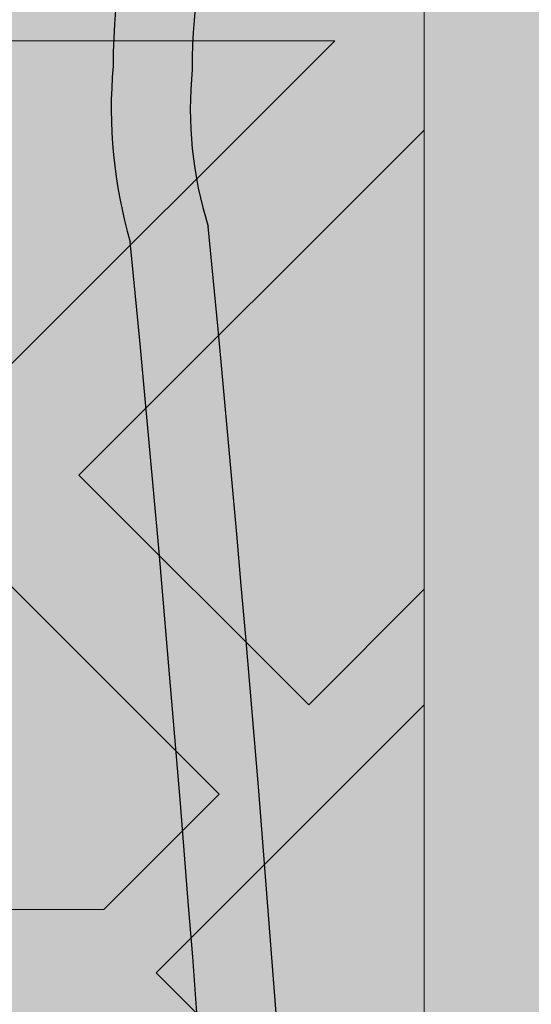
# Model space of a CAD drawing. Units: inches. Extents: x 844 to 2234, y 346 to 1084.
# Tile 20 of 93: x 1126.504 to 1127.536, y 701.258 to 703.246. Entities that reach past the tile are written whole.
import ezdxf

# ---------------------------------------------------------------- set-up
doc = ezdxf.new("R2010")
doc.units = ezdxf.units.IN
doc.header["$MEASUREMENT"] = 0
for name, color, linetype, lineweight in [('A-ANNO-DIMS', 2, 'Continuous', 18), ('furniture', 8, 'Continuous', 18), ('RA-AP-01$0$INT', 35, 'Continuous', 5)]:
    doc.layers.add(name, color=color, linetype=linetype, lineweight=lineweight)
doc.layers.add('RA-AP-01$0$FURN', color=3, linetype='Continuous')
doc.layers.add('RA-AP-01$0$WOOD', color=64, linetype='Continuous')
doc.styles.get("Standard").update_dxf_attribs({"font": 'arial.ttf'})
doc.dimstyles.get("Standard").update_dxf_attribs({"dimtxt": 6, "dimasz": 3, "dimexe": 0.18, "dimexo": 0.0625, "dimgap": 0.09, "dimtad": 0, "dimtih": 1, "dimtoh": 1, "dimdec": 1, "dimzin": 0, "dimdsep": 46, "dimlunit": 3, "dimtxsty": 'Standard', "dimblk": 'ARCHTICK', "dimcen": 0.09, "dimadec": 0, "dimazin": 0, "dimtfac": 1, "dimtdec": 1, "dimtofl": 0, "dimtmove": 0, "dimatfit": 3, "dimfxl": 1, "dimtolj": 1, "dimtzin": 0, "dimarcsym": 0})

# ---------------------------------------------------------------- blocks, each defined once
blk = doc.blocks.new('A$C18D01794')
at = {"layer": 'RA-AP-01$0$INT'}
blk.add_hatch(color=256, dxfattribs=at).paths.add_polyline_path([(4.505206456958071, -7.906712009588039), (5.305206456958072, -7.906712009588039), (5.305206456958072, -7.106712009588038), (5.255206456951893, -7.106712009588036), (5.25520645694868, -7.856712009570104), (4.555206456959269, -7.856712009588616), (4.555206456956052, -7.106712009588038), (4.505206456958073, -7.106712009588038)])
h = blk.add_hatch(color=256, dxfattribs=at)
h.paths.add_polyline_path([(4.585917135068448, -7.856712009587804), (4.614201406330596, -7.856712009587056), (4.668846067270487, -7.802067348644738), (4.723490728212344, -7.856712009584164), (4.771774999457151, -7.856712009582887), (4.826419660396886, -7.80206734864072), (4.862780050090322, -7.838427738332541), (4.844495778842715, -7.856712009580965), (4.862780050090411, -7.856712009580482), (4.905206456960182, -7.814285602707865), (4.947632863832445, -7.856712009578238), (4.965917135079675, -7.856712009577755), (4.947632863831759, -7.838427738330656), (4.983993253523576, -7.802067348637219), (5.038637914464627, -7.856712009575829), (5.08692218571208, -7.856712009574554), (5.141566846649976, -7.802067348634224), (5.196211507589851, -7.856712009571666), (5.224495778822615, -7.856712009570916), (4.905206456953975, -7.537422687702283)])
h.paths.add_polyline_path([(4.895206456956031, -7.575706958950402), (4.895206456958921, -7.684996280828174), (4.840561796018589, -7.630351619890275)], flags=16)
h.paths.add_polyline_path([(4.915206456955638, -7.575706958949956), (4.969851117895509, -7.630351619887399), (4.915206456957609, -7.684996280827732)], flags=16)
h.paths.add_polyline_path([(4.826419660395175, -7.644493755514321), (4.881064321335613, -7.699138416452331), (4.771774999456703, -7.69913841645522)], flags=16)
h.paths.add_polyline_path([(4.983993253519558, -7.644493755510815), (5.038637914460456, -7.699138416449285), (4.929348592581548, -7.69913841645126)], flags=16)
h.paths.add_polyline_path([(4.881064321336025, -7.719138416452334), (4.826419660397532, -7.773783077393256), (4.771774999457062, -7.719138416455217)], flags=16)
h.paths.add_polyline_path([(4.929348592582019, -7.71913841645126), (5.038637914460982, -7.719138416449284), (4.983993253522945, -7.773783077389749)], flags=16)
h.paths.add_polyline_path([(4.895206456960191, -7.733280552075633), (4.895206456962115, -7.806001331460164), (4.876922185715016, -7.824285602708492), (4.840561796021581, -7.787925213016675)], flags=16)
h.paths.add_polyline_path([(4.915206456958487, -7.733280552075187), (4.969851117899527, -7.787925213013798), (4.933490728206909, -7.824285602708034), (4.9152064569598, -7.806001331461736)], flags=16)
h.paths.add_polyline_path([(4.757632863832376, -7.733280552079264), (4.812277524772842, -7.787925213017304), (4.757632863834348, -7.842569873958233)], flags=16)
h.paths.add_polyline_path([(4.737632863832376, -7.73328055207979), (4.737632863834348, -7.842569873958701), (4.682988202893906, -7.787925213020692)], flags=16)
h.paths.add_polyline_path([(5.05278005008503, -7.733280552072701), (5.052780050087917, -7.842569873951664), (4.998135389146995, -7.787925213013169)], flags=16)
h.paths.add_polyline_path([(5.072780050085024, -7.733280552072333), (5.127424711025931, -7.787925213010806), (5.072780050087916, -7.842569873951244)], flags=16)
h.paths.add_polyline_path([(4.935917135072783, -7.506712009583784), (5.255206456948811, -7.826001331459767), (5.255206456948932, -7.797717060211899), (5.200561796010279, -7.743072399273238), (5.255206456949403, -7.688427738334128), (5.25520645694961, -7.640143467086677), (5.200561796009787, -7.585498806146837), (5.236922185702417, -7.549138416454212), (5.255206456949919, -7.56742268770172), (5.255206456949998, -7.549138416454178), (5.212780050078687, -7.506712009583814), (5.25520645695036, -7.464285602712145), (5.255206456950438, -7.446001331464763), (5.236922185702424, -7.464285602712779), (5.200561796009796, -7.427925213020149), (5.255206456950753, -7.373280552079203), (5.25520645695096, -7.324996280834394), (5.200561796010322, -7.270351619893748), (5.255206456951428, -7.215706958952649), (5.255206456951547, -7.187422687705071)])
h.paths.add_polyline_path([(5.042988202883395, -7.42792521302065), (5.097632863823085, -7.373280552080975), (5.097632863822622, -7.482569873959883)], flags=16)
h.paths.add_polyline_path([(5.028846067259663, -7.442067348644384), (5.083490728198774, -7.496712009583504), (4.974201406321001, -7.496712009583035)], flags=16)
h.paths.add_polyline_path([(5.117632863823087, -7.37328055208089), (5.172277524762331, -7.42792521302015), (5.11763286382262, -7.482569873959851)], flags=16)
h.paths.add_polyline_path([(5.08349072819877, -7.516712009582191), (5.028846067259652, -7.571356670521302), (4.974201406320998, -7.516712009582638)], flags=16)
h.paths.add_polyline_path([(5.131774999446817, -7.35913841645716), (5.186419660386065, -7.413783077396415), (5.241064321325782, -7.359138416456712)], flags=17)
h.paths.add_polyline_path([(5.131774999446228, -7.496712009583703), (5.186419660386065, -7.442067348643883), (5.222780050079488, -7.478427738337313), (5.204495778832781, -7.496712009584014)], flags=16)
h.paths.add_polyline_path([(5.097632863822613, -7.530854145205813), (5.097632863823061, -7.640143467084723), (5.042988202883383, -7.585498806145032)], flags=16)
h.paths.add_polyline_path([(5.131774999446899, -7.339138416457162), (5.241064321325809, -7.339138416456712), (5.186419660386591, -7.284493755517479)], flags=17)
h.paths.add_polyline_path([(5.131774999446226, -7.516712009581999), (5.204495778830767, -7.516712009581702), (5.22278005007868, -7.534996280829206), (5.186419660386049, -7.571356670521828)], flags=16)
h.paths.add_polyline_path([(5.11763286382262, -7.530854145205852), (5.17227752476232, -7.585498806145562), (5.117632863823064, -7.64014346708481)], flags=16)
h.paths.add_polyline_path([(5.186419660386069, -7.599640941770585), (5.241064321325754, -7.654285602710281), (5.131774999446791, -7.654285602709814)], flags=16)
h.paths.add_polyline_path([(5.131774999446872, -7.674285602709813), (5.24106432132578, -7.674285602710282), (5.186419660386554, -7.728930263649504)], flags=16)
h.paths.add_polyline_path([(5.255206456951811, -7.126001331467467), (5.255206456951895, -7.106712009588038), (4.555206456956052, -7.106712009588038), (4.555206456956136, -7.12600133146746), (4.905206456953973, -7.476001331465289)])
h.paths.add_polyline_path([(4.983993253513404, -7.368930263651977), (4.92934859257295, -7.314285602713969), (5.03863791445186, -7.314285602711063)], flags=16)
h.paths.add_polyline_path([(4.969851117889988, -7.383072399276016), (4.915206456952556, -7.437717060215906), (4.915206456949648, -7.328427738338133)], flags=16)
h.paths.add_polyline_path([(4.929348592572535, -7.294285602713971), (4.983993253511019, -7.239640941773039), (5.038637914451496, -7.294285602711065)], flags=16)
h.paths.add_polyline_path([(5.052780050074912, -7.280143467087016), (4.998135389134438, -7.225498806148989), (5.052780050072919, -7.170854145208052)], flags=16)
h.paths.add_polyline_path([(5.07278005007491, -7.280143467086489), (5.072780050072918, -7.170854145207579), (5.127424711013374, -7.225498806145578)], flags=16)
h.paths.add_polyline_path([(4.89520645695295, -7.437717060216355), (4.840561796013067, -7.383072399278919), (4.895206456950961, -7.328427738338582)], flags=16)
h.paths.add_polyline_path([(4.915206456948365, -7.280143467090674), (4.915206456946434, -7.207422687704125), (4.933490728192729, -7.18913841645701), (4.969851117886972, -7.225498806149623)], flags=16)
h.paths.add_polyline_path([(4.881064321327021, -7.314285602715054), (4.82641966038902, -7.368930263655506), (4.771774999448108, -7.314285602717047)], flags=16)
h.paths.add_polyline_path([(4.895206456950073, -7.280143467091125), (4.840561796009022, -7.225498806152518), (4.876922185700835, -7.18913841645908), (4.895206456948749, -7.207422687706589)], flags=16)
h.paths.add_polyline_path([(4.983993253510392, -7.211356670525576), (4.947632863816944, -7.174996280833758), (4.965917135064043, -7.156712009585847), (5.038637914448995, -7.156712009584522)], flags=16)
h.paths.add_polyline_path([(4.881064321326543, -7.294285602715056), (4.771774999447578, -7.294285602717046), (4.826419660385607, -7.239640941776569)], flags=16)
h.paths.add_polyline_path([(4.905206456946447, -7.19913841645844), (4.862780050074785, -7.156712009587725), (4.947632863816685, -7.156712009586302)], flags=16)
h.paths.add_polyline_path([(5.14156684663679, -7.211356670521528), (5.086922185696452, -7.156712009583639), (5.196211507574223, -7.156712009581651)], flags=16)
h.paths.add_polyline_path([(4.8264196603837, -7.211356670529104), (4.771774999442643, -7.156712009590501), (4.8444957788276, -7.156712009588568), (4.862780050075511, -7.17499628083566)], flags=16)
h.paths.add_polyline_path([(4.812277524760289, -7.225498806153156), (4.757632863822258, -7.28014346709363), (4.757632863819352, -7.170854145214669)], flags=16)
h.paths.add_polyline_path([(4.73763286382226, -7.280143467093997), (4.682988202881349, -7.22549880615554), (4.737632863819352, -7.170854145215086)], flags=16)
h.paths.add_polyline_path([(4.723490728195188, -7.156712009591787), (4.668846067257299, -7.211356670532127), (4.614201406317417, -7.156712009594693)], flags=16)
h.paths.add_polyline_path([(4.597632863829262, -7.506712009583814), (4.555206456957951, -7.54913841645418), (4.555206456958029, -7.56742268770172), (4.573490728205535, -7.549138416454212), (4.609851117898167, -7.585498806146839), (4.555206456958338, -7.640143467086675), (4.555206456958546, -7.688427738334125), (4.60985111789767, -7.743072399273238), (4.555206456959015, -7.797717060211899), (4.555206456959138, -7.826001331459767), (4.874495778835167, -7.506712009583786), (4.5552064569564, -7.187422687705062), (4.555206456956523, -7.215706958952644), (4.609851117897629, -7.270351619893746), (4.555206456956988, -7.324996280834396), (4.555206456957198, -7.373280552079195), (4.609851117898153, -7.427925213020147), (4.573490728205528, -7.464285602712779), (4.555206456957507, -7.446001331464756), (4.555206456957585, -7.464285602712143)])
h.paths.add_polyline_path([(4.712780050085332, -7.482569873959882), (4.712780050084863, -7.373280552080972), (4.767424711024555, -7.42792521302065)], flags=16)
h.paths.add_polyline_path([(4.726922185709173, -7.496712009583504), (4.781566846648288, -7.442067348644384), (4.836211507586949, -7.496712009583033)], flags=16)
h.paths.add_polyline_path([(4.692780050085327, -7.482569873959851), (4.638135389145619, -7.427925213020149), (4.692780050084865, -7.373280552080892)], flags=16)
h.paths.add_polyline_path([(4.726922185709182, -7.516712009582191), (4.836211507586949, -7.51671200958264), (4.7815668466483, -7.571356670521304)], flags=16)
h.paths.add_polyline_path([(4.678637914461726, -7.496712009583706), (4.605917135075169, -7.496712009584014), (4.587632863828464, -7.478427738337311), (4.623993253521887, -7.442067348643881)], flags=16)
h.paths.add_polyline_path([(4.712780050085336, -7.530854145205816), (4.767424711024568, -7.585498806145034), (4.71278005008489, -7.640143467084724)], flags=16)
h.paths.add_polyline_path([(4.678637914461726, -7.516712009582001), (4.623993253521899, -7.571356670521829), (4.587632863829271, -7.534996280829206), (4.605917135077185, -7.5167120095817)], flags=16)
h.paths.add_polyline_path([(4.692780050085336, -7.530854145205848), (4.692780050084889, -7.64014346708481), (4.638135389145632, -7.585498806145562)], flags=16)
h.paths.add_polyline_path([(4.623993253521885, -7.413783077396415), (4.678637914461131, -7.359138416457161), (4.56934859258217, -7.359138416456712)], flags=17)
h.paths.add_polyline_path([(4.623993253521901, -7.599640941770568), (4.678637914461158, -7.654285602709814), (4.569348592582195, -7.654285602710281)], flags=16)
h.paths.add_polyline_path([(4.678637914461051, -7.339138416457162), (4.623993253521361, -7.284493755517479), (4.569348592582143, -7.339138416456712)], flags=17)
h.paths.add_polyline_path([(4.678637914461076, -7.674285602709813), (4.623993253521399, -7.728930263649504), (4.569348592582167, -7.674285602710281)], flags=16)
h = blk.add_hatch(color=256, dxfattribs=at)
h.paths.add_polyline_path([(5.028846067259997, -7.571356670520955), (4.974201406321342, -7.516712009582294), (5.083490728199115, -7.516712009581846)])
h.paths.add_polyline_path([(4.974201406321344, -7.496712009582688), (5.028846067260004, -7.442067348644037), (5.083490728199117, -7.496712009583157)])
h.paths.add_polyline_path([(5.042988202883738, -7.427925213020309), (5.097632863823428, -7.373280552080627), (5.097632863822963, -7.482569873959537)])
h.paths.add_polyline_path([(5.117632863822961, -7.482569873959509), (5.117632863823428, -7.373280552080546), (5.172277524762674, -7.427925213019804)])
h.paths.add_polyline_path([(5.131774999446572, -7.496712009583358), (5.186419660386406, -7.442067348643536), (5.222780050079831, -7.478427738336961), (5.204495778833122, -7.496712009583667)])
h.paths.add_polyline_path([(5.236922185702764, -7.464285602712433), (5.200561796010139, -7.427925213019802), (5.255206456949971, -7.373280552079975), (5.255206456950271, -7.446001331464927)])
h.paths.add_polyline_path([(5.186419660386412, -7.41378307739607), (5.131774999447164, -7.359138416456815), (5.241064321326123, -7.359138416456366)])
h.paths.add_polyline_path([(5.131774999447238, -7.339138416456815), (5.186419660386934, -7.284493755517132), (5.241064321326153, -7.339138416456368)])
h.paths.add_polyline_path([(5.200561796010663, -7.270351619893402), (5.255206456949324, -7.215706958954747), (5.255206456949777, -7.324996280832518)])
h.paths.add_polyline_path([(5.21278005007903, -7.50671200958347), (5.255206456950223, -7.464285602712278), (5.255206456950696, -7.549138416454185)])
h.paths.add_polyline_path([(5.13177499944657, -7.516712009581652), (5.204495778831106, -7.516712009581354), (5.222780050079024, -7.534996280828858), (5.186419660386397, -7.571356670521485)])
h.paths.add_polyline_path([(5.117632863823405, -7.640143467084465), (5.117632863822955, -7.530854145205498), (5.172277524762665, -7.585498806145217)])
h.paths.add_polyline_path([(5.042988202883727, -7.585498806144689), (5.097632863822957, -7.530854145205474), (5.097632863823407, -7.64014346708438)])
h.paths.add_polyline_path([(5.131774999447135, -7.654285602709467), (5.186419660386394, -7.599640941770219), (5.241064321326097, -7.654285602709933)])
h.paths.add_polyline_path([(5.200561796010128, -7.585498806146492), (5.236922185702758, -7.549138416453866), (5.255206456950264, -7.567422687701371), (5.255206456949948, -7.640143467086325)])
h.paths.add_polyline_path([(5.186419660386895, -7.728930263649157), (5.131774999447213, -7.674285602709467), (5.241064321326127, -7.674285602709934)])
h.paths.add_polyline_path([(5.200561796010624, -7.743072399272893), (5.255206456949745, -7.688427738333778), (5.255206456949276, -7.797717060211553)])
for p, q in [((5.255206456951895, -7.106712009588038), (5.255206456948681, -7.856712009570104)), ((5.212780050078687, -7.506712009583814), (5.25520645694988, -7.464285602712626)), ((5.25520645694988, -7.464285602712626), (5.255206456950353, -7.549138416454534)), ((5.212780050078687, -7.506712009583814), (5.255206456950353, -7.549138416454534)), ((5.204495778831179, -7.5167120095817), (5.131774999446228, -7.516712009581999)), ((5.204495778833082, -7.516712009584017), (5.222780050078681, -7.534996280829206)), ((5.186419660386051, -7.571356670521829), (5.222780050078681, -7.534996280829206)), ((5.200561796009783, -7.585498806146839), (5.236922185702415, -7.549138416454214)), ((5.255206456949919, -7.56742268770172), (5.236922185702415, -7.549138416454212)), ((5.255206456949918, -7.56742268770172), (5.255206456949605, -7.640143467086671)), ((5.255206456949605, -7.640143467086671), (5.200561796009783, -7.585498806146837)), ((5.241064321325755, -7.654285602710281), (5.186419660386049, -7.599640941770568)), ((5.131774999446792, -7.654285602709814), (5.241064321325755, -7.654285602710281))]:
    blk.add_line(p, q, dxfattribs=at)
blk = doc.blocks.new('A$C32926AE1')
at = {"layer": 'RA-AP-01$0$WOOD'}
h = blk.add_hatch(color=256, dxfattribs=at)
h.dxf.hatch_style = 1
h.paths.add_polyline_path([(5.157430609644524, 4.573483066760929, -0.1009492694046607), (5.155401577623758, 4.593365984175333, -0.1842662638101597), (5.172249623284174, 4.638795604568598, 0.2056608120311276), (5.179560981299304, 4.661316324430096, 0.3614336704623542), (5.134352340494423, 4.706524965234944, 0.2056608120311297), (5.111831620632933, 4.699213607219793, -0.1842662638101113), (5.066402000239693, 4.682365561559342, -0.1055311479399994), (5.045656153913092, 4.68467289944697, 0.1567636581983829), (4.763886414745334, 4.684672899446966, -0.1055311479399895), (4.743140568418733, 4.68236556155934, -0.1842662638100833), (4.6977109480255, 4.69921360721979, 0.2056608120302612), (4.675190228164109, 4.706524965234949, 0.3614336704708441), (4.629981587358889, 4.66131632442871, 0.2056608120245944), (4.637292945374126, 4.638795604567974, -0.1842662638101024), (4.654140991034615, 4.59336598417475, -0.1009492694055169), (4.652111959013835, 4.573483066760181, 0.021410119221476), (4.629748025606143, 4.156712009541676, 0.0214101192214795), (4.652111959013809, 3.739940952323101, -0.1009492694059586), (4.654140991034615, 3.720058034908448, -0.1842662638100975), (4.637292945374126, 3.674628414515226, 0.2056608120245705), (4.629981587358889, 3.652107694654492, 0.3614336704708879), (4.675190228164113, 3.606899053848249, 0.2056608120302384), (4.697710948025501, 3.614210411863408, -0.1842662638100995), (4.743140568418738, 3.63105845752386, -0.1055311479402541), (4.763886414745388, 3.628751119636215, 0.1567636581983776), (5.045656153913137, 3.628751119636244, -0.1055311479397538), (5.066402000239692, 3.631058457523857, -0.1842662638101067), (5.111831620632931, 3.614210411863407, 0.2056608120310924), (5.134352340494417, 3.606899053848256, 0.3614336704624001), (5.179560981299307, 3.652107694653103, 0.2056608120311314), (5.172249623284175, 3.6746284145146, -0.1842662638101402), (5.155401577623758, 3.72005803490786, -0.1009492694051366), (5.15743060964455, 3.739940952322354, 0.0214101192215073), (5.179794543052287, 4.156712009541468, 0.0214101192215252)])
h.paths.add_polyline_path([(4.639748609479751, 4.156712009541513, 0.0213537860821624), (4.661970494867118, 3.741887061152232, -0.094075836301374), (4.664143710413708, 3.7196126951003, -0.1824818158568985), (4.644813765429836, 3.668037719127816, 0.2056608120245319), (4.639939526753007, 3.653023905887301, 0.3614336704710246), (4.676106439397173, 3.616856993242342, 0.2056608120302234), (4.691120252638095, 3.621731231919122, -0.1824818158602558), (4.742695228611606, 3.641061176902986, -0.1029891339458722), (4.766991894714349, 3.638256818950944, 0.156709409989566), (5.042550673941472, 3.638256818950105, -0.102989133958497), (5.066847340047078, 3.641061176902949, -0.1824818158594995), (5.118422316020358, 3.621731231919103, 0.2056608120311416), (5.133436129261316, 3.616856993242346, 0.3614336704621468), (5.169603041905217, 3.653023905886178, 0.2056608120310986), (5.164728803228477, 3.668037719127177, -0.1824818158565612), (5.145398858244737, 3.719612695099578, -0.0940758363009313), (5.147572073791232, 3.741887061151398, 0.0213537860822023), (5.169793959178681, 4.156712009541451, 0.0213537860822226), (5.147572073791203, 4.571536957931898, -0.0940758363005034), (5.145398858244737, 4.59381132398362, -0.1824818158565587), (5.164728803228476, 4.645386299956021, 0.2056608120311045), (5.169603041905216, 4.66040011319702, 0.3614336704621845), (5.133436129261313, 4.696567025840856, 0.2056608120310773), (5.118422316020359, 4.691692787164098, -0.182481815859508), (5.066847340047078, 4.67236284218025, -0.1029891339584606), (5.04255067394148, 4.675167200133092, 0.156709409989566), (4.766991894714357, 4.675167200132257, -0.1029891339458842), (4.742695228611611, 4.672362842180213, -0.1824818158602725), (4.691120252638095, 4.691692787164077, 0.2056608120302152), (4.676106439397174, 4.696567025840858, 0.3614336704710363), (4.639939526753005, 4.660400113195899, 0.2056608120245495), (4.644813765429837, 4.645386299955384, -0.1824818158568934), (4.664143710413708, 4.593811323982902, -0.0940758363009187), (4.661970494867149, 4.571536957931074, 0.021353786082177)], flags=16)
h.paths.add_polyline_path([(5.129794543052235, 4.432167055276933, -0.0141661062790638), (5.130152669293814, 4.156927903047693, -0.0141661062790647), (5.129794543052234, 3.881688750818433, -0.0785247771143638), (5.10979738006795, 3.755143611847103, 0.0945969212073497), (5.105408519571111, 3.717898134952927, 0.1043170707844957), (5.116074640131521, 3.670385395016088, 0.1043170707864965), (5.068561900193738, 3.681051515576561, 0.09459692119553), (5.031316423304057, 3.676662655080835, -0.1580239521427272), (4.778226145355827, 3.676662655080367, 0.0945969211986668), (4.740980668464973, 3.681051515576592, 0.1043170707882822), (4.693467928526415, 3.670385395015844, 0.1043170707867916), (4.704134049087309, 3.717898134953662, 0.0945969211972894), (4.69974518859162, 3.755143611844042, -0.0785247771163196), (4.679748025606343, 3.881688750818406, -0.0141661062790663), (4.679389899364763, 4.156927903047693, -0.0141661062790672), (4.679748025606343, 4.432167055276998, -0.0785247771163064), (4.699745188591625, 4.55871219425134, 0.094596921197333), (4.704134049087308, 4.595957671141738, 0.1043170707867205), (4.693467928526416, 4.643470411079523, 0.1043170707882628), (4.740980668464965, 4.632804290518776, 0.0945969211988114), (4.778226145355874, 4.637193151015016, -0.158023952142669), (5.031316423304015, 4.637193151014546, 0.0945969211956361), (5.068561900193736, 4.632804290518806, 0.1043170707864979), (5.11607464013152, 4.643470411079278, 0.1043170707844617), (5.105408519571112, 4.595957671142455, 0.0945969212074597), (5.109797380067959, 4.558712194248236, -0.0785247771143467)], flags=0)
h.paths.add_polyline_path([(5.119794532311105, 4.432259799204851, -0.0142000800617244), (5.120156169157484, 4.156927903047701, -0.0142000800617277), (5.119794532311105, 3.881596006890482, -0.0784894509520253), (5.100273383573699, 3.758192358677797, 0.0940138827242913), (5.095413455884425, 3.717477693979438, 0.0606271852308753), (5.099615656341024, 3.686844378806616, 0.0606271852322524), (5.068982341167493, 3.691046579263239, 0.0940138827010453), (5.028267676478798, 3.686186651576848, -0.1580706864508061), (4.781274892180912, 3.686186651576435, 0.0940138827026903), (4.740560227491556, 3.691046579263279, 0.0606271852339895), (4.709926912317155, 3.686844378806508, 0.0606271852329405), (4.714129112773991, 3.717477693980356, 0.094013882701304), (4.709269185087677, 3.758192358669163, -0.0784894509577193), (4.689748036347473, 3.881596006890469, -0.014200080061729), (4.689386399501094, 4.156927903047709, -0.0142000800617217), (4.689748036347473, 4.432259799204808, -0.078489450957724), (4.709269185087651, 4.555663447426125, 0.0940138827014585), (4.714129112773992, 4.596378112114996, 0.0606271852329731), (4.709926912317154, 4.62701142728886, 0.0606271852340196), (4.74056022749157, 4.622809226832087, 0.0940138827024997), (4.781274892180847, 4.627669154518912, -0.1580706864508359), (5.028267676478777, 4.627669154518526, 0.0940138827010946), (5.068982341167492, 4.622809226832129, 0.060627185232254), (5.099615656341024, 4.627011427288751, 0.0606271852308727), (5.095413455884425, 4.59637811211593, 0.0940138827241088), (5.100273383573675, 4.555663447417647, -0.0784894509520978)], flags=0)
h.paths.add_polyline_path([(5.06978912287499, 4.430218106756144, -0.014241683694547), (5.070173729147532, 4.156927903047672, -0.0142416836945458), (5.06978912287499, 3.883637699339223, -0.0800609523125196), (5.052662118612511, 3.773463122773442, 0.0526421978001116), (5.04590916754064, 3.740550867606997, 0.0526421977992423), (5.012996912374707, 3.73379791653534, -0.1583028414718258), (4.796545656286308, 3.73379791653451, 0.0526421978034211), (4.763633401117837, 3.740550867607021, 0.0526421978018622), (4.756880450045755, 3.773463122774558, -0.0800609523117106), (4.739753445783639, 3.883637699339268, -0.0142416836945435), (4.739368839511098, 4.156927903047671, -0.0142416836945477), (4.739753445783639, 4.430218106756155, -0.0800609523116345), (4.75688045004574, 4.540392683320762, 0.052642197801941), (4.763633401117837, 4.573304938488346, 0.0526421978035071), (4.796545656286361, 4.580057889560873, -0.1583028414717561), (5.012996912374669, 4.580057889560039, 0.0526421977993048), (5.04590916754064, 4.57330493848837, 0.0526421978002057), (5.052662118612529, 4.540392683321868, -0.080060952312477)], flags=0)
h.paths.add_polyline_path([(5.049789715110557, 4.43038092723357, -0.0143097550741839), (5.05018085590259, 4.156927903047715, -0.0143097550741854), (5.049789715110558, 3.883474878861827, -0.0800685599149176), (5.03362098255317, 3.779581877367999, 0.0306258898956367), (5.028241146483733, 3.758218888663947, 0.0306258898977031), (5.006878157778253, 3.75283905259408, -0.1583983521624096), (4.802664410878162, 3.752839052594731, 0.0306258898946014), (4.781301422174808, 3.758218888663924, 0.0306258898967912), (4.775921586105202, 3.779581877368794, -0.080068559914251), (4.759752853548071, 3.883474878861786, -0.0143097550741854), (4.759361712756037, 4.156927903047671, -0.0143097550741854), (4.759752853548071, 4.430380927233557, -0.0800685599142479), (4.775921586105193, 4.534273928726546, 0.0306258898968306), (4.781301422174808, 4.555636917431444, 0.0306258898945754), (4.802664410878143, 4.561016753500631, -0.1583983521624168), (5.006878157778244, 4.561016753501291, 0.0306258898977177), (5.028241146483733, 4.555636917431421, 0.0306258898958182), (5.03362098255321, 4.534273928727244, -0.080068559914796)], flags=0)
h.paths.add_polyline_path([(4.999766070382627, 4.428171244713864, -0.0143443147609634), (5.000198441819402, 4.156927903047689, -0.0143443147609612), (4.999766070382627, 3.885684561381556, -0.0784641635803329), (4.987356730658798, 3.799103304488872, -0.1506053783831347), (4.822185837999821, 3.79910330448882, -0.0784641635803318), (4.809776498276007, 3.885684561381509, -0.014344314760963), (4.809344126839227, 4.156927903047677, -0.0143443147609645), (4.809776498276007, 4.428171244713873, -0.0784641635803192), (4.822185837999822, 4.514752501606549, -0.1506053783831338), (4.987356730658798, 4.514752501606494, -0.078464163580285)], flags=0)
h.paths.add_polyline_path([(4.979755254238824, 4.42764379880488, -0.0143772539198268), (4.980205517789977, 4.156927903047693, -0.0143772539198275), (4.979755254238824, 3.886212007290489, -0.0689242507424422), (4.971183264704897, 3.815276770442801, -0.1296645318904179), (4.838359303953726, 3.815276770442746, -0.0689242507424186), (4.829787314419809, 3.886212007290419, -0.0143772539198292), (4.829337050868653, 4.156927903047653, -0.0143772539198325), (4.829787314419809, 4.427643798804946, -0.0689242507424211), (4.838359303953725, 4.498579035652621, -0.1296645318904187), (4.971183264704897, 4.498579035652565, -0.0689242507424401)], flags=0)
h = blk.add_hatch(color=256, dxfattribs=at)
h.dxf.hatch_style = 1
h.paths.add_polyline_path([(5.145398858244737, 4.59381132398362, -0.1824818158565616), (5.164728803228476, 4.645386299956021, 0.2056608120311045), (5.169603041905216, 4.66040011319702, 0.3614336704621845), (5.133436129261313, 4.696567025840856, 0.2056608120310773), (5.118422316020359, 4.691692787164098, -0.182481815859508), (5.066847340047078, 4.67236284218025, -0.1029891339584606), (5.04255067394148, 4.675167200133092, 0.156709409989566), (4.766991894714357, 4.675167200132257, -0.1029891339458842), (4.742695228611611, 4.672362842180213, -0.1824818158602725), (4.691120252638095, 4.691692787164077, 0.2056608120302152), (4.676106439397174, 4.696567025840858, 0.3614336704710363), (4.639939526753005, 4.660400113195899, 0.2056608120245495), (4.644813765429837, 4.645386299955384, -0.1824818158568934), (4.664143710413708, 4.593811323982902, -0.0940758363009187), (4.661970494867149, 4.571536957931074, 0.0213537860821772), (4.639748609479751, 4.156712009541507, 0.0213537860821625), (4.661970494867119, 3.741887061152226, -0.0940758363013071), (4.664143710413708, 3.719612695100309, -0.1824818158569294), (4.644813765429836, 3.668037719127816, 0.2056608120245319), (4.639939526753007, 3.653023905887301, 0.3614336704710246), (4.676106439397173, 3.616856993242342, 0.2056608120302234), (4.691120252638095, 3.621731231919122, -0.1824818158602558), (4.742695228611606, 3.641061176902986, -0.1029891339458722), (4.766991894714349, 3.638256818950944, 0.156709409989566), (5.042550673941472, 3.638256818950105, -0.102989133958497), (5.066847340047078, 3.641061176902949, -0.1824818158594995), (5.118422316020358, 3.621731231919103, 0.2056608120311416), (5.133436129261316, 3.616856993242346, 0.3614336704621468), (5.169603041905217, 3.653023905886178, 0.2056608120310986), (5.164728803228477, 3.668037719127177, -0.1824818158565612), (5.145398858244737, 3.719612695099578, -0.0940758363009313), (5.147572073791232, 3.741887061151398, 0.0213537860822023), (5.169793959178681, 4.156712009541451, 0.0213537860822226), (5.147572073791203, 4.571536957931898, -0.0940758363004996)])
h.paths.add_polyline_path([(5.109797380067958, 4.55871219424824, -0.0785247771143472), (5.129794543052234, 4.432167055276936, -0.0141661062790644), (5.130152669293814, 4.156927903047685, -0.014166106279066), (5.129794543052234, 3.881688750818401, -0.0785247771143517), (5.109797380067946, 3.755143611847092, 0.0945969212073132), (5.105408519571111, 3.717898134952929, 0.1043170707844995), (5.116074640131521, 3.670385395016088, 0.1043170707864965), (5.068561900193738, 3.681051515576561, 0.09459692119553), (5.031316423304057, 3.676662655080835, -0.1580239521427272), (4.778226145355827, 3.676662655080367, 0.0945969211986668), (4.740980668464973, 3.681051515576592, 0.1043170707882822), (4.693467928526415, 3.670385395015844, 0.1043170707867916), (4.704134049087309, 3.717898134953662, 0.0945969211972894), (4.69974518859162, 3.755143611844042, -0.0785247771163196), (4.679748025606343, 3.881688750818406, -0.0141661062790663), (4.679389899364763, 4.156927903047693, -0.0141661062790672), (4.679748025606343, 4.432167055276998, -0.0785247771163064), (4.699745188591625, 4.55871219425134, 0.094596921197333), (4.704134049087308, 4.595957671141738, 0.1043170707867205), (4.693467928526416, 4.643470411079523, 0.1043170707882628), (4.740980668464965, 4.632804290518776, 0.0945969211988114), (4.778226145355874, 4.637193151015016, -0.158023952142669), (5.031316423304015, 4.637193151014546, 0.0945969211956361), (5.068561900193736, 4.632804290518806, 0.1043170707864979), (5.11607464013152, 4.643470411079278, 0.1043170707844617), (5.105408519571112, 4.595957671142455, 0.0945969212074504)], flags=16)
h.paths.add_polyline_path([(5.100273383573655, 4.55566344741771, -0.0784894509521388), (5.119794532311105, 4.432259799204852, -0.0142000800617252), (5.120156169157484, 4.156927903047686, -0.014200080061726), (5.119794532311105, 3.881596006890502, -0.0784894509520446), (5.100273383573696, 3.758192358677786, 0.0940138827242721), (5.095413455884425, 3.717477693979436, 0.0606271852308692), (5.099615656341024, 3.686844378806616, 0.0606271852322522), (5.068982341167493, 3.691046579263239, 0.0940138827010453), (5.028267676478798, 3.686186651576848, -0.1580706864508061), (4.781274892180912, 3.686186651576435, 0.0940138827026903), (4.740560227491556, 3.691046579263279, 0.0606271852339895), (4.709926912317155, 3.686844378806508, 0.0606271852329405), (4.714129112773991, 3.717477693980356, 0.094013882701304), (4.709269185087677, 3.758192358669163, -0.0784894509577193), (4.689748036347473, 3.881596006890469, -0.014200080061729), (4.689386399501094, 4.156927903047709, -0.0142000800617217), (4.689748036347473, 4.432259799204808, -0.078489450957724), (4.709269185087651, 4.555663447426125, 0.0940138827014585), (4.714129112773992, 4.596378112114996, 0.0606271852329731), (4.709926912317154, 4.62701142728886, 0.0606271852340196), (4.74056022749157, 4.622809226832087, 0.0940138827024997), (4.781274892180847, 4.627669154518912, -0.1580706864508359), (5.028267676478777, 4.627669154518526, 0.0940138827010946), (5.068982341167492, 4.622809226832129, 0.060627185232254), (5.099615656341024, 4.627011427288751, 0.0606271852308727), (5.095413455884425, 4.59637811211593, 0.094013882723957)], flags=0)
h.paths.add_polyline_path([(5.04590916754064, 4.57330493848837, 0.0526421978002057), (5.052662118612529, 4.540392683321868, -0.0800609523124783), (5.06978912287499, 4.430218106756142, -0.0142416836945469), (5.070173729147532, 4.156927903047672, -0.0142416836945458), (5.06978912287499, 3.883637699339223, -0.0800609523125196), (5.052662118612511, 3.773463122773442, 0.0526421978001116), (5.04590916754064, 3.740550867606997, 0.0526421977992423), (5.012996912374707, 3.73379791653534, -0.1583028414718258), (4.796545656286308, 3.73379791653451, 0.0526421978034211), (4.763633401117837, 3.740550867607021, 0.0526421978018622), (4.756880450045755, 3.773463122774558, -0.0800609523117106), (4.739753445783639, 3.883637699339268, -0.0142416836945435), (4.739368839511098, 4.156927903047671, -0.0142416836945477), (4.739753445783639, 4.430218106756155, -0.0800609523116345), (4.75688045004574, 4.540392683320762, 0.052642197801941), (4.763633401117837, 4.573304938488346, 0.0526421978035071), (4.796545656286361, 4.580057889560873, -0.1583028414717561), (5.012996912374669, 4.580057889560039, 0.0526421977993048)], flags=0)
h.paths.add_polyline_path([(5.028241146483733, 4.555636917431422, 0.0306258898956949), (5.033620982553182, 4.534273928727329, -0.0800685599148649), (5.049789715110557, 4.430380927233569, -0.0143097550741839), (5.05018085590259, 4.156927903047715, -0.0143097550741854), (5.049789715110558, 3.883474878861827, -0.0800685599149176), (5.03362098255317, 3.779581877367999, 0.0306258898956367), (5.028241146483733, 3.758218888663947, 0.0306258898977031), (5.006878157778253, 3.75283905259408, -0.1583983521624096), (4.802664410878162, 3.752839052594731, 0.0306258898946014), (4.781301422174808, 3.758218888663924, 0.0306258898967912), (4.775921586105202, 3.779581877368794, -0.080068559914251), (4.759752853548071, 3.883474878861786, -0.0143097550741854), (4.759361712756037, 4.156927903047671, -0.0143097550741854), (4.759752853548071, 4.430380927233557, -0.0800685599142479), (4.775921586105193, 4.534273928726546, 0.0306258898968306), (4.781301422174808, 4.555636917431444, 0.0306258898945754), (4.802664410878143, 4.561016753500631, -0.1583983521624168), (5.006878157778244, 4.561016753501291, 0.0306258898977174)], flags=0)
h.paths.add_polyline_path([(4.987356730658798, 4.514752501606494, -0.0784641635803018), (4.999766070382627, 4.428171244713845, -0.0143443147609637), (5.000198441819402, 4.156927903047665, -0.0143443147609622), (4.999766070382628, 3.885684561381514, -0.0784641635802952), (4.987356730658797, 3.799103304488872, -0.1506053783831338), (4.822185837999821, 3.799103304488819, -0.0784641635803342), (4.809776498276007, 3.885684561381512, -0.0143443147609628), (4.809344126839227, 4.156927903047676, -0.0143443147609646), (4.809776498276007, 4.428171244713873, -0.0784641635803192), (4.822185837999822, 4.514752501606549, -0.1506053783831338)], flags=0)
h.paths.add_polyline_path([(4.971183264704897, 4.498579035652566, -0.0689242507424384), (4.979755254238824, 4.427643798804883, -0.0143772539198276), (4.980205517789977, 4.15692790304768, -0.0143772539198258), (4.979755254238823, 3.88621200729051, -0.0689242507424628), (4.971183264704897, 3.815276770442801, -0.129664531890417), (4.838359303953726, 3.815276770442746, -0.0689242507424186), (4.829787314419809, 3.886212007290419, -0.0143772539198292), (4.829337050868653, 4.156927903047653, -0.0143772539198325), (4.829787314419809, 4.427643798804946, -0.0689242507424211), (4.838359303953725, 4.498579035652621, -0.1296645318904187)], flags=0)
for centre, radius, start, end in [((5.223368649208389, 4.593998637499738), 0.0779700159629894, 138.7710509204691, 180.1376463004422), ((5.223368649208353, 4.593998637499641), 0.067970015963027, 138.7710509203988, 180.5333070514128), ((5.205154176610212, 4.588398198542794), 0.0599999999999777, 174.823807838761, 196.3211313301264), ((5.205154176610233, 4.588398198542771), 0.0500000000000019, 174.2979292346878, 197.3556839753019), ((0.304323780376417, 4.104079819130551), 4.875754844654793, 0.6185013483537143, 5.524589681839913), ((0.304323780376417, 4.104079819130551), 4.865754844654794, 0.6185013483537143, 5.512956158076888)]:
    blk.add_arc(centre, radius, start, end, dxfattribs=at)
blk = doc.blocks.new('A$C5D2F253E')
at = {"layer": 'RA-AP-01$0$FURN', "xscale": -0.7999999999883585, "yscale": 0.7999999999883585, "zscale": 0.8, "rotation": 90}
blk.add_blockref('A$C18D01794', (-5.687757199772477, 4.75791982714071), dxfattribs=at)
at = {"layer": 'RA-AP-01$0$WOOD', "rotation": 270}
blk.add_blockref('A$C32926AE1', (-4.161339601644158, 5.73852594588169), dxfattribs=at)
blk = doc.blocks.new('_ArchTick')
at = {"color": 0, "linetype": 'ByBlock', "const_width": 0.15}
blk.add_lwpolyline([(-0.5, -0.5), (0.5, 0.5)], dxfattribs=at)
blk = doc.blocks.new('*D144')
at = {"layer": 'A-ANNO-DIMS', "color": 0, "lineweight": -2, "transparency": 16777216}
for p, q in [((1096.615948, 439.3732739999999), (1096.615948, 1074.743301)), ((1143.115948, 492.373274), (1143.115948, 1074.743301)), ((1096.615948, 1074.563301), (1102.481950728513, 1074.563301)), ((1143.115948, 1074.563301), (1137.249945271487, 1074.563301))]:
    blk.add_line(p, q, dxfattribs=at)
at = {"layer": 'Defpoints', "color": 0, "transparency": 16777216}
for p in [(1143.115948, 1074.563301), (1143.115948, 492.3107739999999), (1096.615948, 439.3107739999999)]:
    blk.add_point(p, dxfattribs=at)
at = {"layer": 'A-ANNO-DIMS', "color": 0, "lineweight": -2, "transparency": 16777216, "xscale": 3, "yscale": 3, "zscale": 3, "rotation": 180}
blk.add_blockref('_ArchTick', (1096.615948, 1074.563301), dxfattribs=at)
at = {"layer": 'A-ANNO-DIMS', "color": 0, "lineweight": -2, "transparency": 16777216, "xscale": 3, "yscale": 3, "zscale": 3}
blk.add_blockref('_ArchTick', (1143.115948, 1074.563301), dxfattribs=at)
at = {"layer": 'A-ANNO-DIMS', "color": 0, "transparency": 16777216, "insert": (1119.865948, 1074.563301), "char_height": 6, "attachment_point": 5}
blk.add_mtext('\\A1;3\'-10 1/2"', dxfattribs=at)

msp = doc.modelspace()

# ---------------------------------------------------------------- block references
at = {"layer": 'furniture', "xscale": 15.94108302203742, "yscale": 15.94108302203742, "zscale": 15.94108302203742, "rotation": 90}
msp.add_blockref('A$C5D2F253E', (1136.147844094663, 696.2584716700112), dxfattribs=at)

# ---------------------------------------------------------------- dimensions: what is measured, and where the dimension line sits
at = {"layer": 'A-ANNO-DIMS'}
dim = msp.add_linear_dim(base=(1143.115948, 1074.563301), p1=(1096.615948, 439.3107739999999), p2=(1143.115948, 492.3107739999999), dimstyle='Standard', override={"dimdec": 1, "dimlfac": 1, "dimrnd": 0, "dimzin": 1, "dimdsep": 46, "dimlunit": 4, "dimfrac": 2}, dxfattribs=at)
dim.commit()
dim.dimension.update_dxf_attribs({"geometry": '*D144', "text_midpoint": (1119.865948, 1074.563301)})

doc.saveas('drawing.dxf')
